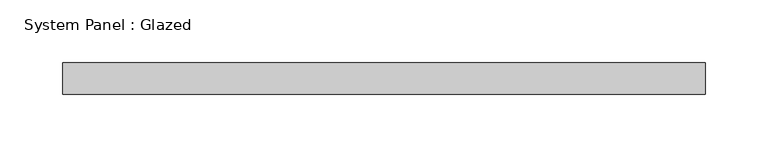
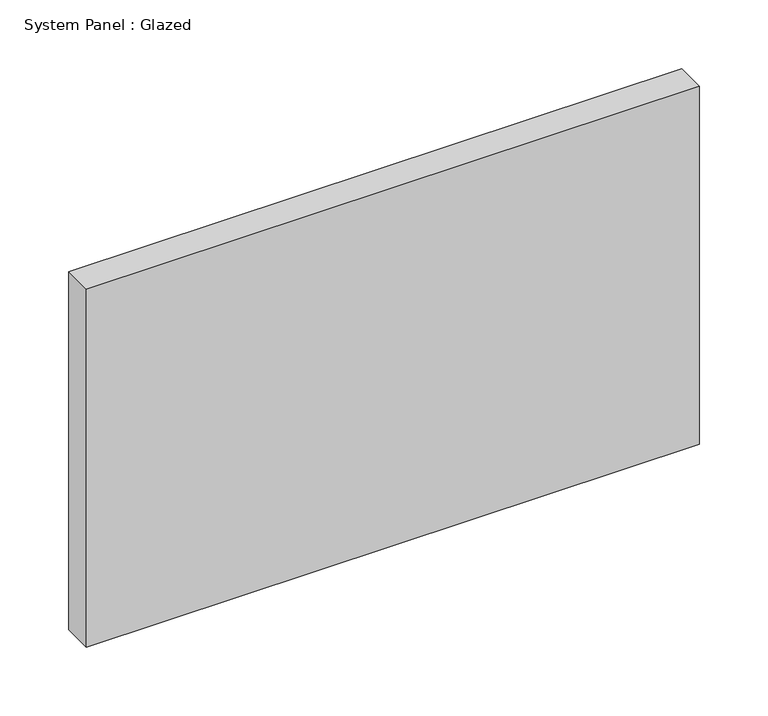
"""IFC4 building model written with IfcOpenShell, lengths in millimetres: plate geometry, System Panel : Glazed."""

from ifc_helpers import new_model, si_unit, origin, origin_with_axes, place, context, project, spatial, polyline, outline, extrude, source, transform, mapped, element, save


def system_panel_glazed_f6df7fa7(model_context):
    return source(origin(), model_context, "Body", "SweptSolid", [
        extrude(outline(polyline([(257.175, 19.05), (-257.175, 19.05), (-257.175, 44.45), (257.175, 44.45), (257.175, 19.05)])), origin_with_axes(), (0.0, 0.0, 1.0), 317.5),
    ])


if __name__ == "__main__":
    model = new_model("IFC4")
    model_context = context("Model", 3, world=origin())
    ifc_project = project(units=[si_unit("LENGTHUNIT", "METRE", prefix="MILLI")], contexts=[model_context])
    site = spatial("IfcSite", under=ifc_project)
    building = spatial("IfcBuilding", under=site)
    placement = place(None, origin())
    system_panel_glazed_shape = system_panel_glazed_f6df7fa7(model_context)
    element("IfcPlate", 1, ObjectType="System Panel : Glazed", at=placement, inside=building, context=model_context, shape_type="MappedRepresentation", body=[
        mapped(system_panel_glazed_shape, transform((0.0, 0.0, 0.0), x_axis=(1.0, 0.0, 0.0), y_axis=(0.0, 1.0, 0.0), z_axis=(0.0, 0.0, 1.0))),
    ])
    save(model, "model.ifc")

# Revit data of these elements
# Type "System Panel : Glazed"
#   Construction Type Id = "GSP4R"
#   Analytic Construction = "1/8 in Pilkington single glazing"
#   Visual Light Transmittance = 0.9
#   Solar Heat Gain Coefficient = 0.86
#   Heat Transfer Coefficient (U) = 1.18115 BTU/(h·ft²·°F)
#   Define Thermal Properties by = 1
# Element 1 (IfcPlate, "System Panel : Glazed")
#   Materials on its faces: "Glass"
# Materials
#   "Glass": class "Glass", colour RGB 0 128 192, transparency 0.75, Description = "Soda Lime Glass", Cost = 0
